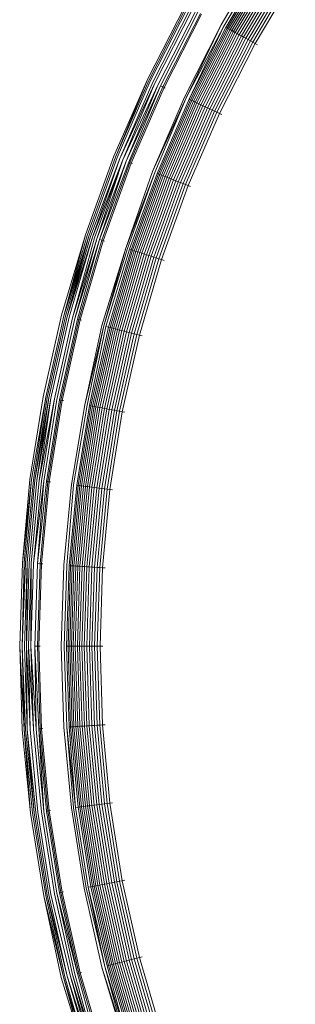
# Model space of a CAD drawing. Units: inches. Extents: x 64 to 1167, y 117 to 939.
# Tile 43 of 56: x 1129.1267 to 1129.3597, y 500.6393 to 501.4737. Entities that reach past the tile are written whole.
import ezdxf

# ---------------------------------------------------------------- set-up
doc = ezdxf.new("R2010")
doc.units = ezdxf.units.IN
doc.header["$MEASUREMENT"] = 0
doc.layers.add('A-FLOR-FIXT', color=8, linetype='Continuous', lineweight=18)

msp = doc.modelspace()

# ---------------------------------------------------------------- linework, layer by layer
at = {"layer": 'A-FLOR-FIXT'}
for p, q in [((1129.33193, 501.5286), (1129.29696, 501.46948)), ((1129.33413, 501.5272), (1129.29925, 501.46822)), ((1129.33586, 501.52611), (1129.30104, 501.46724)), ((1129.33689, 501.52546), (1129.30211, 501.46665)), ((1129.33802, 501.52474), (1129.30328, 501.466)), ((1129.33926, 501.52395), (1129.30457, 501.46529)), ((1129.34059, 501.52311), (1129.30595, 501.46453)), ((1129.34201, 501.5222), (1129.30743, 501.46372)), ((1129.34352, 501.52125), (1129.30899, 501.46286)), ((1129.34511, 501.52024), (1129.31064, 501.46196)), ((1129.34676, 501.51919), (1129.31236, 501.46101)), ((1129.34848, 501.5181), (1129.31414, 501.46003)), ((1129.35026, 501.51697), (1129.31599, 501.45902)), ((1129.35208, 501.51581), (1129.31788, 501.45798)), ((1129.35395, 501.51463), (1129.31982, 501.45691)), ((1129.35585, 501.51342), (1129.32179, 501.45583)), ((1129.35777, 501.5122), (1129.32378, 501.45473)), ((1129.35971, 501.51097), (1129.3258, 501.45362)), ((1129.2668, 501.48606), (1129.23464, 501.42293)), ((1129.26805, 501.48537), (1129.23593, 501.42232)), ((1129.26918, 501.48475), (1129.23709, 501.42177)), ((1129.27125, 501.48361), (1129.23923, 501.42076)), ((1129.27285, 501.48273), (1129.24089, 501.41999)), ((1129.27553, 501.48126), (1129.24365, 501.41869)), ((1129.27744, 501.48021), (1129.24562, 501.41776)), ((1129.27943, 501.47912), (1129.24767, 501.41679)), ((1129.28043, 501.47856), (1129.24871, 501.4163)), ((1129.29696, 501.46948), (1129.26598, 501.40818)), ((1129.29696, 501.46948), (1129.2674, 501.40751)), ((1129.29925, 501.46822), (1129.2674, 501.40751)), ((1129.29925, 501.46822), (1129.26998, 501.40629)), ((1129.30104, 501.46724), (1129.26998, 501.40629)), ((1129.30211, 501.46665), (1129.27109, 501.40577)), ((1129.30328, 501.466), (1129.27231, 501.4052)), ((1129.30457, 501.46529), (1129.27363, 501.40458)), ((1129.30595, 501.46453), (1129.27506, 501.4039)), ((1129.30211, 501.46665), (1129.30104, 501.46724)), ((1129.30328, 501.466), (1129.30211, 501.46665)), ((1129.30457, 501.46529), (1129.30328, 501.466)), ((1129.30595, 501.46453), (1129.30457, 501.46529)), ((1129.30743, 501.46372), (1129.30595, 501.46453)), ((1129.30743, 501.46372), (1129.27658, 501.40319)), ((1129.30899, 501.46286), (1129.2782, 501.40243)), ((1129.31064, 501.46196), (1129.2799, 501.40163)), ((1129.31236, 501.46101), (1129.28167, 501.40079)), ((1129.31414, 501.46003), (1129.28352, 501.39992)), ((1129.31599, 501.45902), (1129.28542, 501.39903)), ((1129.31788, 501.45798), (1129.28738, 501.39811)), ((1129.31982, 501.45691), (1129.28937, 501.39717)), ((1129.32179, 501.45583), (1129.29141, 501.39621)), ((1129.30899, 501.46286), (1129.30743, 501.46372)), ((1129.31064, 501.46196), (1129.30899, 501.46286)), ((1129.31236, 501.46101), (1129.31064, 501.46196)), ((1129.31414, 501.46003), (1129.31236, 501.46101)), ((1129.31599, 501.45902), (1129.31414, 501.46003)), ((1129.31788, 501.45798), (1129.31599, 501.45902)), ((1129.31982, 501.45691), (1129.31788, 501.45798)), ((1129.32179, 501.45583), (1129.31982, 501.45691)), ((1129.32378, 501.45473), (1129.32179, 501.45583)), ((1129.32378, 501.45473), (1129.29347, 501.39524)), ((1129.3258, 501.45362), (1129.29555, 501.39426)), ((1129.3258, 501.45362), (1129.32378, 501.45473)), ((1129.32782, 501.45251), (1129.3258, 501.45362)), ((1129.23464, 501.42293), (1129.20619, 501.35802)), ((1129.23464, 501.42293), (1129.20782, 501.35737)), ((1129.23593, 501.42232), (1129.20782, 501.35737)), ((1129.23709, 501.42177), (1129.20902, 501.3569)), ((1129.23923, 501.42076), (1129.21122, 501.35603)), ((1129.24089, 501.41999), (1129.21122, 501.35603)), ((1129.24089, 501.41999), (1129.21383, 501.355)), ((1129.24365, 501.41869), (1129.21383, 501.355)), ((1129.24365, 501.41869), (1129.21676, 501.35384)), ((1129.24562, 501.41776), (1129.21676, 501.35384)), ((1129.24562, 501.41776), (1129.21883, 501.35302)), ((1129.24767, 501.41679), (1129.21989, 501.3526)), ((1129.24871, 501.4163), (1129.22096, 501.35217)), ((1129.24767, 501.41679), (1129.24562, 501.41776)), ((1129.24767, 501.41679), (1129.24871, 501.4163)), ((1129.24871, 501.4163), (1129.24976, 501.41581)), ((1129.26598, 501.40818), (1129.23905, 501.34501)), ((1129.2674, 501.40751), (1129.23905, 501.34501)), ((1129.2674, 501.40751), (1129.24092, 501.34427)), ((1129.26998, 501.40629), (1129.24282, 501.34352)), ((1129.27109, 501.40577), (1129.24395, 501.34307)), ((1129.27109, 501.40577), (1129.26998, 501.40629)), ((1129.27231, 501.4052), (1129.27109, 501.40577)), ((1129.27231, 501.4052), (1129.2452, 501.34257)), ((1129.27363, 501.40458), (1129.24657, 501.34203)), ((1129.27506, 501.4039), (1129.24803, 501.34145)), ((1129.27658, 501.40319), (1129.2496, 501.34083)), ((1129.2782, 501.40243), (1129.25126, 501.34018)), ((1129.2799, 501.40163), (1129.25301, 501.33948)), ((1129.28167, 501.40079), (1129.25483, 501.33876)), ((1129.28352, 501.39992), (1129.25672, 501.33801)), ((1129.28542, 501.39903), (1129.25868, 501.33724)), ((1129.28738, 501.39811), (1129.26069, 501.33644)), ((1129.28937, 501.39717), (1129.26274, 501.33563)), ((1129.27363, 501.40458), (1129.27231, 501.4052)), ((1129.27506, 501.4039), (1129.27363, 501.40458)), ((1129.27658, 501.40319), (1129.27506, 501.4039)), ((1129.2782, 501.40243), (1129.27658, 501.40319)), ((1129.2799, 501.40163), (1129.2782, 501.40243)), ((1129.28167, 501.40079), (1129.2799, 501.40163)), ((1129.28352, 501.39992), (1129.28167, 501.40079)), ((1129.28542, 501.39903), (1129.28352, 501.39992)), ((1129.28738, 501.39811), (1129.28542, 501.39903)), ((1129.28937, 501.39717), (1129.28738, 501.39811)), ((1129.29141, 501.39621), (1129.28937, 501.39717)), ((1129.29141, 501.39621), (1129.26484, 501.3348)), ((1129.29347, 501.39524), (1129.26695, 501.33396)), ((1129.29555, 501.39426), (1129.26909, 501.33312)), ((1129.29347, 501.39524), (1129.29141, 501.39621)), ((1129.29555, 501.39426), (1129.29347, 501.39524)), ((1129.29764, 501.39328), (1129.29555, 501.39426)), ((1129.20619, 501.35802), (1129.18218, 501.29134)), ((1129.20782, 501.35737), (1129.18385, 501.29079)), ((1129.20902, 501.3569), (1129.18507, 501.2904)), ((1129.21122, 501.35603), (1129.18652, 501.28993)), ((1129.21122, 501.35603), (1129.18817, 501.28939)), ((1129.21383, 501.355), (1129.18817, 501.28939)), ((1129.21383, 501.355), (1129.19, 501.2888)), ((1129.21383, 501.355), (1129.19197, 501.28816)), ((1129.21676, 501.35384), (1129.19197, 501.28816)), ((1129.21676, 501.35384), (1129.19404, 501.28748)), ((1129.21883, 501.35302), (1129.19404, 501.28748)), ((1129.21989, 501.3526), (1129.1962, 501.28678)), ((1129.22096, 501.35217), (1129.19729, 501.28643)), ((1129.21883, 501.35302), (1129.21989, 501.3526)), ((1129.21989, 501.3526), (1129.22096, 501.35217)), ((1129.22096, 501.35217), (1129.22203, 501.35175)), ((1129.23905, 501.34501), (1129.2163, 501.28025)), ((1129.24092, 501.34427), (1129.2163, 501.28025)), ((1129.24092, 501.34427), (1129.21771, 501.27979)), ((1129.24282, 501.34352), (1129.21965, 501.27916)), ((1129.24395, 501.34307), (1129.22081, 501.27879)), ((1129.2452, 501.34257), (1129.22209, 501.27837)), ((1129.24657, 501.34203), (1129.22348, 501.27792)), ((1129.24803, 501.34145), (1129.22498, 501.27743)), ((1129.2496, 501.34083), (1129.22659, 501.27691)), ((1129.25126, 501.34018), (1129.22829, 501.27636)), ((1129.25301, 501.33948), (1129.23007, 501.27578)), ((1129.25483, 501.33876), (1129.23194, 501.27517)), ((1129.24282, 501.34352), (1129.24395, 501.34307)), ((1129.24395, 501.34307), (1129.2452, 501.34257)), ((1129.2452, 501.34257), (1129.24657, 501.34203)), ((1129.24657, 501.34203), (1129.24803, 501.34145)), ((1129.24803, 501.34145), (1129.2496, 501.34083)), ((1129.2496, 501.34083), (1129.25126, 501.34018)), ((1129.25126, 501.34018), (1129.25301, 501.33948)), ((1129.25301, 501.33948), (1129.25483, 501.33876)), ((1129.25483, 501.33876), (1129.25672, 501.33801)), ((1129.25672, 501.33801), (1129.23387, 501.27454)), ((1129.25868, 501.33724), (1129.23587, 501.27389)), ((1129.26069, 501.33644), (1129.23793, 501.27322)), ((1129.26274, 501.33563), (1129.24003, 501.27254)), ((1129.26484, 501.3348), (1129.24217, 501.27185)), ((1129.26695, 501.33396), (1129.24434, 501.27114)), ((1129.26909, 501.33312), (1129.24652, 501.27043)), ((1129.25672, 501.33801), (1129.25868, 501.33724)), ((1129.25868, 501.33724), (1129.26069, 501.33644)), ((1129.26069, 501.33644), (1129.26274, 501.33563)), ((1129.26274, 501.33563), (1129.26484, 501.3348)), ((1129.26484, 501.3348), (1129.26695, 501.33396)), ((1129.26695, 501.33396), (1129.26909, 501.33312)), ((1129.26909, 501.33312), (1129.27124, 501.33227)), ((1129.18218, 501.29134), (1129.16197, 501.22339)), ((1129.18218, 501.29134), (1129.16411, 501.22284)), ((1129.18385, 501.29079), (1129.16411, 501.22284)), ((1129.18507, 501.2904), (1129.16411, 501.22284)), ((1129.18507, 501.2904), (1129.16535, 501.22252)), ((1129.18507, 501.2904), (1129.16683, 501.22214)), ((1129.18652, 501.28993), (1129.16683, 501.22214)), ((1129.18817, 501.28939), (1129.16683, 501.22214)), ((1129.18817, 501.28939), (1129.16851, 501.22171)), ((1129.19, 501.2888), (1129.17135, 501.22098)), ((1129.19197, 501.28816), (1129.17135, 501.22098)), ((1129.19197, 501.28816), (1129.17342, 501.22045)), ((1129.19404, 501.28748), (1129.17342, 501.22045)), ((1129.19404, 501.28748), (1129.17558, 501.21989)), ((1129.1962, 501.28678), (1129.17668, 501.21961)), ((1129.19729, 501.28643), (1129.1778, 501.21933)), ((1129.1962, 501.28678), (1129.19404, 501.28748)), ((1129.19729, 501.28643), (1129.1962, 501.28678)), ((1129.19839, 501.28607), (1129.19729, 501.28643)), ((1129.2163, 501.28025), (1129.19606, 501.21464)), ((1129.2163, 501.28025), (1129.1978, 501.21419)), ((1129.21771, 501.27979), (1129.1978, 501.21419)), ((1129.21965, 501.27916), (1129.19951, 501.21375)), ((1129.22081, 501.27879), (1129.20175, 501.21318)), ((1129.22209, 501.27837), (1129.20305, 501.21284)), ((1129.22348, 501.27792), (1129.20447, 501.21248)), ((1129.22498, 501.27743), (1129.206, 501.21208)), ((1129.22659, 501.27691), (1129.20763, 501.21166)), ((1129.22829, 501.27636), (1129.20936, 501.21122)), ((1129.23007, 501.27578), (1129.21118, 501.21075)), ((1129.23194, 501.27517), (1129.21308, 501.21027)), ((1129.23387, 501.27454), (1129.21505, 501.20976)), ((1129.23587, 501.27389), (1129.21709, 501.20924)), ((1129.23793, 501.27322), (1129.21918, 501.2087)), ((1129.22081, 501.27879), (1129.21965, 501.27916)), ((1129.22209, 501.27837), (1129.22081, 501.27879)), ((1129.24003, 501.27254), (1129.22132, 501.20815)), ((1129.22348, 501.27792), (1129.22209, 501.27837)), ((1129.22498, 501.27743), (1129.22348, 501.27792)), ((1129.22659, 501.27691), (1129.22498, 501.27743)), ((1129.22829, 501.27636), (1129.22659, 501.27691)), ((1129.23007, 501.27578), (1129.22829, 501.27636)), ((1129.23194, 501.27517), (1129.23007, 501.27578)), ((1129.23387, 501.27454), (1129.23194, 501.27517)), ((1129.23587, 501.27389), (1129.23387, 501.27454)), ((1129.23793, 501.27322), (1129.23587, 501.27389)), ((1129.24003, 501.27254), (1129.23793, 501.27322)), ((1129.24217, 501.27185), (1129.24003, 501.27254)), ((1129.24217, 501.27185), (1129.2235, 501.20759)), ((1129.24434, 501.27114), (1129.22571, 501.20702)), ((1129.24652, 501.27043), (1129.22794, 501.20645)), ((1129.24434, 501.27114), (1129.24217, 501.27185)), ((1129.24652, 501.27043), (1129.24434, 501.27114)), ((1129.24872, 501.26972), (1129.24652, 501.27043)), ((1129.16197, 501.22339), (1129.1465, 501.15419)), ((1129.16411, 501.22284), (1129.14867, 501.15378)), ((1129.16535, 501.22252), (1129.14993, 501.15354)), ((1129.16683, 501.22214), (1129.15143, 501.15325)), ((1129.16851, 501.22171), (1129.15313, 501.15293)), ((1129.17135, 501.22098), (1129.15602, 501.15238)), ((1129.17342, 501.22045), (1129.15811, 501.15198)), ((1129.17558, 501.21989), (1129.1603, 501.15156)), ((1129.17668, 501.21961), (1129.16142, 501.15135)), ((1129.1778, 501.21933), (1129.16255, 501.15113)), ((1129.17668, 501.21961), (1129.17558, 501.21989)), ((1129.1778, 501.21933), (1129.17668, 501.21961)), ((1129.17891, 501.21904), (1129.1778, 501.21933)), ((1129.19606, 501.21464), (1129.18167, 501.14749)), ((1129.1978, 501.21419), (1129.18167, 501.14749)), ((1129.1978, 501.21419), (1129.18364, 501.14711)), ((1129.19951, 501.21375), (1129.18565, 501.14673)), ((1129.20175, 501.21318), (1129.19951, 501.21375)), ((1129.20175, 501.21318), (1129.18684, 501.1465)), ((1129.20305, 501.21284), (1129.18817, 501.14625)), ((1129.20447, 501.21248), (1129.18961, 501.14597)), ((1129.206, 501.21208), (1129.19116, 501.14568)), ((1129.20763, 501.21166), (1129.19281, 501.14536)), ((1129.20936, 501.21122), (1129.19457, 501.14503)), ((1129.21118, 501.21075), (1129.19641, 501.14467)), ((1129.21308, 501.21027), (1129.19834, 501.14431)), ((1129.21505, 501.20976), (1129.20034, 501.14392)), ((1129.20305, 501.21284), (1129.20175, 501.21318)), ((1129.21709, 501.20924), (1129.2024, 501.14353)), ((1129.20447, 501.21248), (1129.20305, 501.21284)), ((1129.206, 501.21208), (1129.20447, 501.21248)), ((1129.21918, 501.2087), (1129.20453, 501.14313)), ((1129.20763, 501.21166), (1129.206, 501.21208)), ((1129.22132, 501.20815), (1129.2067, 501.14271)), ((1129.20936, 501.21122), (1129.20763, 501.21166)), ((1129.2235, 501.20759), (1129.20891, 501.14229)), ((1129.21118, 501.21075), (1129.20936, 501.21122)), ((1129.22571, 501.20702), (1129.21114, 501.14186)), ((1129.21308, 501.21027), (1129.21118, 501.21075)), ((1129.21505, 501.20976), (1129.21308, 501.21027)), ((1129.22794, 501.20645), (1129.2134, 501.14143)), ((1129.21709, 501.20924), (1129.21505, 501.20976)), ((1129.21918, 501.2087), (1129.21709, 501.20924)), ((1129.22132, 501.20815), (1129.21918, 501.2087)), ((1129.2235, 501.20759), (1129.22132, 501.20815)), ((1129.22571, 501.20702), (1129.2235, 501.20759)), ((1129.22794, 501.20645), (1129.22571, 501.20702)), ((1129.23017, 501.20588), (1129.22794, 501.20645)), ((1129.1465, 501.15419), (1129.1353, 501.08418)), ((1129.14867, 501.15378), (1129.13659, 501.08401)), ((1129.14867, 501.15378), (1129.13821, 501.08381)), ((1129.14993, 501.15354), (1129.1396, 501.08363)), ((1129.15143, 501.15325), (1129.1396, 501.08363)), ((1129.15143, 501.15325), (1129.14122, 501.08343)), ((1129.15313, 501.15293), (1129.14122, 501.08343)), ((1129.15313, 501.15293), (1129.14304, 501.0832)), ((1129.15602, 501.15238), (1129.14304, 501.0832)), ((1129.15602, 501.15238), (1129.14502, 501.08295)), ((1129.15811, 501.15198), (1129.14714, 501.08268)), ((1129.1603, 501.15156), (1129.14935, 501.0824)), ((1129.16142, 501.15135), (1129.15048, 501.08226)), ((1129.16255, 501.15113), (1129.15162, 501.08212)), ((1129.1603, 501.15156), (1129.16142, 501.15135)), ((1129.16142, 501.15135), (1129.16255, 501.15113)), ((1129.16255, 501.15113), (1129.16369, 501.15092)), ((1129.18167, 501.14749), (1129.17056, 501.07972)), ((1129.18364, 501.14711), (1129.17211, 501.07953)), ((1129.18565, 501.14673), (1129.17495, 501.07917)), ((1129.18684, 501.1465), (1129.17616, 501.07902)), ((1129.18817, 501.14625), (1129.17749, 501.07885)), ((1129.18961, 501.14597), (1129.17894, 501.07866)), ((1129.19116, 501.14568), (1129.18051, 501.07847)), ((1129.19281, 501.14536), (1129.18218, 501.07825)), ((1129.19457, 501.14503), (1129.18395, 501.07803)), ((1129.18684, 501.1465), (1129.18565, 501.14673)), ((1129.19641, 501.14467), (1129.18582, 501.0778)), ((1129.18817, 501.14625), (1129.18684, 501.1465)), ((1129.19834, 501.14431), (1129.18776, 501.07755)), ((1129.18961, 501.14597), (1129.18817, 501.14625)), ((1129.19116, 501.14568), (1129.18961, 501.14597)), ((1129.20034, 501.14392), (1129.18978, 501.07729)), ((1129.19281, 501.14536), (1129.19116, 501.14568)), ((1129.2024, 501.14353), (1129.19187, 501.07703)), ((1129.19457, 501.14503), (1129.19281, 501.14536)), ((1129.20453, 501.14313), (1129.19401, 501.07676)), ((1129.19641, 501.14467), (1129.19457, 501.14503)), ((1129.2067, 501.14271), (1129.19621, 501.07648)), ((1129.19834, 501.14431), (1129.19641, 501.14467)), ((1129.20034, 501.14392), (1129.19834, 501.14431)), ((1129.20891, 501.14229), (1129.19844, 501.0762)), ((1129.2024, 501.14353), (1129.20034, 501.14392)), ((1129.21114, 501.14186), (1129.2007, 501.07592)), ((1129.20453, 501.14313), (1129.2024, 501.14353)), ((1129.2134, 501.14143), (1129.20298, 501.07563)), ((1129.2067, 501.14271), (1129.20453, 501.14313)), ((1129.20891, 501.14229), (1129.2067, 501.14271)), ((1129.21114, 501.14186), (1129.20891, 501.14229)), ((1129.2134, 501.14143), (1129.21114, 501.14186)), ((1129.21567, 501.141), (1129.2134, 501.14143)), ((1129.1353, 501.08418), (1129.12892, 501.01356)), ((1129.13659, 501.08401), (1129.12892, 501.01356)), ((1129.13659, 501.08401), (1129.1304, 501.01347)), ((1129.13821, 501.08381), (1129.13155, 501.0134)), ((1129.1396, 501.08363), (1129.13296, 501.01331)), ((1129.14122, 501.08343), (1129.13459, 501.01321)), ((1129.14304, 501.0832), (1129.13641, 501.01309)), ((1129.14502, 501.08295), (1129.13841, 501.01297)), ((1129.14714, 501.08268), (1129.13841, 501.01297)), ((1129.14714, 501.08268), (1129.14164, 501.01276)), ((1129.14935, 501.0824), (1129.14164, 501.01276)), ((1129.15048, 501.08226), (1129.1439, 501.01262)), ((1129.15162, 501.08212), (1129.14505, 501.01255)), ((1129.15048, 501.08226), (1129.14935, 501.0824)), ((1129.15162, 501.08212), (1129.15048, 501.08226)), ((1129.15277, 501.08197), (1129.15162, 501.08212)), ((1129.17056, 501.07972), (1129.16409, 501.01135)), ((1129.17211, 501.07953), (1129.16647, 501.0112)), ((1129.17495, 501.07917), (1129.16851, 501.01107)), ((1129.17616, 501.07902), (1129.16973, 501.011)), ((1129.17749, 501.07885), (1129.17107, 501.01091)), ((1129.17894, 501.07866), (1129.17253, 501.01082)), ((1129.18051, 501.07847), (1129.17411, 501.01072)), ((1129.17616, 501.07902), (1129.17495, 501.07917)), ((1129.18218, 501.07825), (1129.17579, 501.01062)), ((1129.17749, 501.07885), (1129.17616, 501.07902)), ((1129.17894, 501.07866), (1129.17749, 501.07885)), ((1129.18395, 501.07803), (1129.17757, 501.0105)), ((1129.18051, 501.07847), (1129.17894, 501.07866)), ((1129.18582, 501.0778), (1129.17944, 501.01039)), ((1129.18218, 501.07825), (1129.18051, 501.07847)), ((1129.18776, 501.07755), (1129.1814, 501.01026)), ((1129.18395, 501.07803), (1129.18218, 501.07825)), ((1129.18978, 501.07729), (1129.18344, 501.01013)), ((1129.18582, 501.0778), (1129.18395, 501.07803)), ((1129.19187, 501.07703), (1129.18553, 501.01)), ((1129.18776, 501.07755), (1129.18582, 501.0778)), ((1129.19401, 501.07676), (1129.18769, 501.00987)), ((1129.18978, 501.07729), (1129.18776, 501.07755)), ((1129.19187, 501.07703), (1129.18978, 501.07729)), ((1129.19621, 501.07648), (1129.1899, 501.00973)), ((1129.19187, 501.07703), (1129.19401, 501.07676)), ((1129.19844, 501.0762), (1129.19214, 501.00959)), ((1129.19401, 501.07676), (1129.19621, 501.07648)), ((1129.2007, 501.07592), (1129.19442, 501.00944)), ((1129.19621, 501.07648), (1129.19844, 501.0762)), ((1129.20298, 501.07563), (1129.19671, 501.0093)), ((1129.19844, 501.0762), (1129.2007, 501.07592)), ((1129.2007, 501.07592), (1129.20298, 501.07563)), ((1129.20298, 501.07563), (1129.20527, 501.07534)), ((1129.12892, 501.01356), (1129.1267, 500.94271)), ((1129.1304, 501.01347), (1129.12872, 500.94271)), ((1129.13155, 501.0134), (1129.12872, 500.94271)), ((1129.13296, 501.01331), (1129.13074, 500.94271)), ((1129.13296, 501.01331), (1129.13237, 500.94271)), ((1129.13459, 501.01321), (1129.13237, 500.94271)), ((1129.13641, 501.01309), (1129.1342, 500.94271)), ((1129.13641, 501.01309), (1129.1362, 500.94271)), ((1129.13841, 501.01297), (1129.1362, 500.94271)), ((1129.14164, 501.01276), (1129.13944, 500.94271)), ((1129.14164, 501.01276), (1129.1439, 501.01262)), ((1129.1439, 501.01262), (1129.1417, 500.94271)), ((1129.14505, 501.01255), (1129.14285, 500.94271)), ((1129.1439, 501.01262), (1129.14505, 501.01255)), ((1129.14505, 501.01255), (1129.1462, 501.01248)), ((1129.16409, 501.01135), (1129.16171, 500.94271)), ((1129.16647, 501.0112), (1129.16432, 500.94271)), ((1129.16851, 501.01107), (1129.16636, 500.94271)), ((1129.16973, 501.011), (1129.16758, 500.94271)), ((1129.16973, 501.011), (1129.16851, 501.01107)), ((1129.17107, 501.01091), (1129.16893, 500.94271)), ((1129.17107, 501.01091), (1129.16973, 501.011)), ((1129.17253, 501.01082), (1129.17039, 500.94271)), ((1129.17253, 501.01082), (1129.17107, 501.01091)), ((1129.17411, 501.01072), (1129.17197, 500.94271)), ((1129.17411, 501.01072), (1129.17253, 501.01082)), ((1129.17579, 501.01062), (1129.17366, 500.94271)), ((1129.17579, 501.01062), (1129.17411, 501.01072)), ((1129.17757, 501.0105), (1129.17544, 500.94271)), ((1129.17757, 501.0105), (1129.17579, 501.01062)), ((1129.17944, 501.01039), (1129.17732, 500.94271)), ((1129.17944, 501.01039), (1129.17757, 501.0105)), ((1129.1814, 501.01026), (1129.17928, 500.94271)), ((1129.1814, 501.01026), (1129.17944, 501.01039)), ((1129.18344, 501.01013), (1129.18132, 500.94271)), ((1129.18344, 501.01013), (1129.1814, 501.01026)), ((1129.18553, 501.01), (1129.18342, 500.94271)), ((1129.18553, 501.01), (1129.18344, 501.01013)), ((1129.18769, 501.00987), (1129.18553, 501.01)), ((1129.18769, 501.00987), (1129.18558, 500.94271)), ((1129.1899, 501.00973), (1129.18769, 501.00987)), ((1129.1899, 501.00973), (1129.18779, 500.94271)), ((1129.19214, 501.00959), (1129.1899, 501.00973)), ((1129.19214, 501.00959), (1129.19004, 500.94271)), ((1129.19442, 501.00944), (1129.19214, 501.00959)), ((1129.19442, 501.00944), (1129.19232, 500.94271)), ((1129.19671, 501.0093), (1129.19442, 501.00944)), ((1129.19671, 501.0093), (1129.19462, 500.94271)), ((1129.19901, 501.00915), (1129.19671, 501.0093)), ((1129.1267, 500.94271), (1129.1304, 500.87194)), ((1129.1267, 500.94271), (1129.12874, 500.87184)), ((1129.12872, 500.94271), (1129.1304, 500.87194)), ((1129.12872, 500.94271), (1129.13155, 500.87202)), ((1129.13074, 500.94271), (1129.13296, 500.87211)), ((1129.13237, 500.94271), (1129.13548, 500.87226)), ((1129.13237, 500.94271), (1129.13296, 500.87211)), ((1129.1342, 500.94271), (1129.13841, 500.87245)), ((1129.1342, 500.94271), (1129.13548, 500.87226)), ((1129.1362, 500.94271), (1129.14054, 500.87258)), ((1129.1362, 500.94271), (1129.13841, 500.87245)), ((1129.1417, 500.94271), (1129.13944, 500.94271)), ((1129.13944, 500.94271), (1129.14276, 500.87272)), ((1129.13944, 500.94271), (1129.14054, 500.87258)), ((1129.14285, 500.94271), (1129.1417, 500.94271)), ((1129.1417, 500.94271), (1129.1439, 500.87279)), ((1129.144, 500.94271), (1129.14285, 500.94271)), ((1129.14285, 500.94271), (1129.14505, 500.87287)), ((1129.16171, 500.94271), (1129.16387, 500.87405)), ((1129.16432, 500.94271), (1129.16647, 500.87421)), ((1129.16636, 500.94271), (1129.16758, 500.94271)), ((1129.16636, 500.94271), (1129.16851, 500.87434)), ((1129.16758, 500.94271), (1129.16893, 500.94271)), ((1129.16758, 500.94271), (1129.16973, 500.87442)), ((1129.16893, 500.94271), (1129.17039, 500.94271)), ((1129.16893, 500.94271), (1129.17107, 500.8745)), ((1129.17039, 500.94271), (1129.17197, 500.94271)), ((1129.17039, 500.94271), (1129.17253, 500.8746)), ((1129.17197, 500.94271), (1129.17366, 500.94271)), ((1129.17197, 500.94271), (1129.17411, 500.87469)), ((1129.17366, 500.94271), (1129.17544, 500.94271)), ((1129.17366, 500.94271), (1129.17579, 500.8748)), ((1129.17544, 500.94271), (1129.17732, 500.94271)), ((1129.17544, 500.94271), (1129.17757, 500.87491)), ((1129.17732, 500.94271), (1129.17928, 500.94271)), ((1129.17732, 500.94271), (1129.17944, 500.87503)), ((1129.17928, 500.94271), (1129.18132, 500.94271)), ((1129.17928, 500.94271), (1129.1814, 500.87515)), ((1129.18132, 500.94271), (1129.18342, 500.94271)), ((1129.18132, 500.94271), (1129.18344, 500.87528)), ((1129.18342, 500.94271), (1129.18558, 500.94271)), ((1129.18342, 500.94271), (1129.18553, 500.87541)), ((1129.18558, 500.94271), (1129.18769, 500.87555)), ((1129.18558, 500.94271), (1129.18779, 500.94271)), ((1129.18779, 500.94271), (1129.19004, 500.94271)), ((1129.18779, 500.94271), (1129.1899, 500.87569)), ((1129.19004, 500.94271), (1129.19232, 500.94271)), ((1129.19004, 500.94271), (1129.19214, 500.87583)), ((1129.19232, 500.94271), (1129.19462, 500.94271)), ((1129.19232, 500.94271), (1129.19442, 500.87597)), ((1129.19462, 500.94271), (1129.19693, 500.94271)), ((1129.19462, 500.94271), (1129.19671, 500.87612)), ((1129.12874, 500.87184), (1129.13586, 500.80131)), ((1129.1304, 500.87194), (1129.1376, 500.80153)), ((1129.1304, 500.87194), (1129.13586, 500.80131)), ((1129.13155, 500.87202), (1129.13888, 500.80169)), ((1129.13296, 500.87211), (1129.13888, 500.80169)), ((1129.13296, 500.87211), (1129.14039, 500.80188)), ((1129.13548, 500.87226), (1129.14211, 500.8021)), ((1129.13841, 500.87245), (1129.14502, 500.80247)), ((1129.14054, 500.87258), (1129.14714, 500.80273)), ((1129.14276, 500.87272), (1129.1439, 500.87279)), ((1129.14276, 500.87272), (1129.14935, 500.80301)), ((1129.14276, 500.87272), (1129.14714, 500.80273)), ((1129.1439, 500.87279), (1129.14505, 500.87287)), ((1129.1439, 500.87279), (1129.15048, 500.80316)), ((1129.14505, 500.87287), (1129.1462, 500.87294)), ((1129.14505, 500.87287), (1129.15162, 500.8033)), ((1129.16387, 500.87405), (1129.17056, 500.80569)), ((1129.16647, 500.87421), (1129.17387, 500.80611)), ((1129.16647, 500.87421), (1129.17211, 500.80589)), ((1129.16973, 500.87442), (1129.16851, 500.87434)), ((1129.16851, 500.87434), (1129.17387, 500.80611)), ((1129.17107, 500.8745), (1129.16973, 500.87442)), ((1129.16973, 500.87442), (1129.17616, 500.8064)), ((1129.17253, 500.8746), (1129.17107, 500.8745)), ((1129.17107, 500.8745), (1129.17749, 500.80657)), ((1129.17411, 500.87469), (1129.17253, 500.8746)), ((1129.17253, 500.8746), (1129.17894, 500.80675)), ((1129.17579, 500.8748), (1129.17411, 500.87469)), ((1129.17411, 500.87469), (1129.18051, 500.80695)), ((1129.17757, 500.87491), (1129.17579, 500.8748)), ((1129.17579, 500.8748), (1129.18218, 500.80716)), ((1129.17944, 500.87503), (1129.17757, 500.87491)), ((1129.17757, 500.87491), (1129.18395, 500.80738)), ((1129.1814, 500.87515), (1129.17944, 500.87503)), ((1129.17944, 500.87503), (1129.18582, 500.80762)), ((1129.18344, 500.87528), (1129.1814, 500.87515)), ((1129.1814, 500.87515), (1129.18776, 500.80787)), ((1129.18553, 500.87541), (1129.18344, 500.87528)), ((1129.18344, 500.87528), (1129.18978, 500.80812)), ((1129.18769, 500.87555), (1129.18553, 500.87541)), ((1129.18553, 500.87541), (1129.19187, 500.80838)), ((1129.1899, 500.87569), (1129.18769, 500.87555)), ((1129.18769, 500.87555), (1129.19401, 500.80865)), ((1129.19214, 500.87583), (1129.1899, 500.87569)), ((1129.1899, 500.87569), (1129.19621, 500.80893)), ((1129.19442, 500.87597), (1129.19214, 500.87583)), ((1129.19214, 500.87583), (1129.19844, 500.80921)), ((1129.19671, 500.87612), (1129.19442, 500.87597)), ((1129.19442, 500.87597), (1129.2007, 500.8095)), ((1129.19901, 500.87626), (1129.19671, 500.87612)), ((1129.19671, 500.87612), (1129.20298, 500.80979)), ((1129.17056, 500.80569), (1129.18108, 500.73782)), ((1129.17211, 500.80589), (1129.18284, 500.73815)), ((1129.17616, 500.8064), (1129.17387, 500.80611)), ((1129.17387, 500.80611), (1129.18458, 500.73848)), ((1129.17749, 500.80657), (1129.17616, 500.8064)), ((1129.17616, 500.8064), (1129.18684, 500.73892)), ((1129.17894, 500.80675), (1129.17749, 500.80657)), ((1129.17749, 500.80657), (1129.18817, 500.73917)), ((1129.18051, 500.80695), (1129.17894, 500.80675)), ((1129.17894, 500.80675), (1129.18961, 500.73944)), ((1129.18218, 500.80716), (1129.18051, 500.80695)), ((1129.18051, 500.80695), (1129.19116, 500.73974)), ((1129.18395, 500.80738), (1129.18218, 500.80716)), ((1129.18218, 500.80716), (1129.19281, 500.74006)), ((1129.18582, 500.80762), (1129.18395, 500.80738)), ((1129.18395, 500.80738), (1129.19457, 500.74039)), ((1129.18776, 500.80787), (1129.18582, 500.80762)), ((1129.18582, 500.80762), (1129.19641, 500.74074)), ((1129.18978, 500.80812), (1129.18776, 500.80787)), ((1129.18776, 500.80787), (1129.19834, 500.74111)), ((1129.19187, 500.80838), (1129.18978, 500.80812)), ((1129.18978, 500.80812), (1129.20034, 500.74149)), ((1129.19401, 500.80865), (1129.19187, 500.80838)), ((1129.19187, 500.80838), (1129.2024, 500.74189)), ((1129.19621, 500.80893), (1129.19401, 500.80865)), ((1129.19401, 500.80865), (1129.20453, 500.74229)), ((1129.19844, 500.80921), (1129.19621, 500.80893)), ((1129.19621, 500.80893), (1129.2067, 500.7427)), ((1129.2007, 500.8095), (1129.19844, 500.80921)), ((1129.19844, 500.80921), (1129.20891, 500.74313)), ((1129.20298, 500.80979), (1129.2007, 500.8095)), ((1129.2007, 500.8095), (1129.21114, 500.74355)), ((1129.20527, 500.81008), (1129.20298, 500.80979)), ((1129.20298, 500.80979), (1129.2134, 500.74398)), ((1129.13586, 500.80131), (1129.14694, 500.73131)), ((1129.1376, 500.80153), (1129.14867, 500.73164)), ((1129.13888, 500.80169), (1129.14993, 500.73188)), ((1129.14039, 500.80188), (1129.15143, 500.73216)), ((1129.14211, 500.8021), (1129.15313, 500.73249)), ((1129.14502, 500.80247), (1129.15602, 500.73304)), ((1129.14714, 500.80273), (1129.15811, 500.73344)), ((1129.15048, 500.80316), (1129.14935, 500.80301)), ((1129.14935, 500.80301), (1129.1603, 500.73385)), ((1129.15162, 500.8033), (1129.15048, 500.80316)), ((1129.15048, 500.80316), (1129.16142, 500.73407)), ((1129.15277, 500.80344), (1129.15162, 500.8033)), ((1129.15162, 500.8033), (1129.16255, 500.73428)), ((1129.18284, 500.73815), (1129.19859, 500.67143)), ((1129.18684, 500.73892), (1129.18458, 500.73848)), ((1129.18458, 500.73848), (1129.20057, 500.67194)), ((1129.18458, 500.73848), (1129.19859, 500.67143)), ((1129.18817, 500.73917), (1129.18684, 500.73892)), ((1129.18684, 500.73892), (1129.20175, 500.67224)), ((1129.18961, 500.73944), (1129.18817, 500.73917)), ((1129.18817, 500.73917), (1129.20305, 500.67257)), ((1129.19116, 500.73974), (1129.18961, 500.73944)), ((1129.18961, 500.73944), (1129.20447, 500.67294)), ((1129.19281, 500.74006), (1129.19116, 500.73974)), ((1129.19116, 500.73974), (1129.206, 500.67333)), ((1129.19457, 500.74039), (1129.19281, 500.74006)), ((1129.19281, 500.74006), (1129.20763, 500.67375)), ((1129.19641, 500.74074), (1129.19457, 500.74039)), ((1129.19457, 500.74039), (1129.20936, 500.67419)), ((1129.19834, 500.74111), (1129.19641, 500.74074)), ((1129.19641, 500.74074), (1129.21118, 500.67466)), ((1129.20034, 500.74149), (1129.19834, 500.74111)), ((1129.19834, 500.74111), (1129.21308, 500.67515)), ((1129.2024, 500.74189), (1129.20034, 500.74149)), ((1129.20034, 500.74149), (1129.21505, 500.67566)), ((1129.20453, 500.74229), (1129.2024, 500.74189)), ((1129.2024, 500.74189), (1129.21709, 500.67618)), ((1129.2067, 500.7427), (1129.20453, 500.74229)), ((1129.20453, 500.74229), (1129.21918, 500.67672)), ((1129.20891, 500.74313), (1129.2067, 500.7427)), ((1129.2067, 500.7427), (1129.22132, 500.67727)), ((1129.21114, 500.74355), (1129.20891, 500.74313)), ((1129.20891, 500.74313), (1129.2235, 500.67783)), ((1129.2134, 500.74398), (1129.21114, 500.74355)), ((1129.21114, 500.74355), (1129.22571, 500.67839)), ((1129.21567, 500.74442), (1129.2134, 500.74398)), ((1129.2134, 500.74398), (1129.22794, 500.67896)), ((1129.14694, 500.73131), (1129.16358, 500.66244)), ((1129.14694, 500.73131), (1129.16182, 500.66199)), ((1129.14867, 500.73164), (1129.16358, 500.66244)), ((1129.14993, 500.73188), (1129.16683, 500.66327)), ((1129.14993, 500.73188), (1129.1647, 500.66273)), ((1129.15143, 500.73216), (1129.16683, 500.66327)), ((1129.15313, 500.73249), (1129.16942, 500.66394)), ((1129.15602, 500.73304), (1129.17135, 500.66444)), ((1129.15811, 500.73344), (1129.17558, 500.66552)), ((1129.15811, 500.73344), (1129.17342, 500.66497)), ((1129.1603, 500.73385), (1129.16142, 500.73407)), ((1129.1603, 500.73385), (1129.17558, 500.66552)), ((1129.16142, 500.73407), (1129.16255, 500.73428)), ((1129.16142, 500.73407), (1129.17668, 500.6658)), ((1129.16255, 500.73428), (1129.16369, 500.7345)), ((1129.16255, 500.73428), (1129.1778, 500.66609)), ((1129.18108, 500.73782), (1129.19606, 500.67078)), ((1129.19859, 500.67143), (1129.21862, 500.60592)), ((1129.19859, 500.67143), (1129.21694, 500.60537)), ((1129.20175, 500.67224), (1129.20057, 500.67194)), ((1129.20057, 500.67194), (1129.21862, 500.60592)), ((1129.20305, 500.67257), (1129.20175, 500.67224)), ((1129.20175, 500.67224), (1129.22081, 500.60663)), ((1129.20447, 500.67294), (1129.20305, 500.67257)), ((1129.20305, 500.67257), (1129.22209, 500.60705)), ((1129.206, 500.67333), (1129.20447, 500.67294)), ((1129.20447, 500.67294), (1129.22348, 500.6075)), ((1129.20763, 500.67375), (1129.206, 500.67333)), ((1129.206, 500.67333), (1129.22498, 500.60799)), ((1129.20936, 500.67419), (1129.20763, 500.67375)), ((1129.20763, 500.67375), (1129.22659, 500.60851)), ((1129.21118, 500.67466), (1129.20936, 500.67419)), ((1129.20936, 500.67419), (1129.22829, 500.60906)), ((1129.21308, 500.67515), (1129.21118, 500.67466)), ((1129.21118, 500.67466), (1129.23007, 500.60964)), ((1129.21505, 500.67566), (1129.21308, 500.67515)), ((1129.21308, 500.67515), (1129.23194, 500.61024)), ((1129.21709, 500.67618), (1129.21505, 500.67566)), ((1129.21505, 500.67566), (1129.23387, 500.61087)), ((1129.21918, 500.67672), (1129.21709, 500.67618)), ((1129.21709, 500.67618), (1129.23587, 500.61152)), ((1129.22132, 500.67727), (1129.21918, 500.67672)), ((1129.21918, 500.67672), (1129.23793, 500.61219)), ((1129.2235, 500.67783), (1129.22132, 500.67727)), ((1129.22132, 500.67727), (1129.24003, 500.61288)), ((1129.22571, 500.67839), (1129.2235, 500.67783)), ((1129.2235, 500.67783), (1129.24217, 500.61357)), ((1129.22794, 500.67896), (1129.22571, 500.67839)), ((1129.22571, 500.67839), (1129.24434, 500.61427)), ((1129.23017, 500.67954), (1129.22794, 500.67896)), ((1129.22794, 500.67896), (1129.24652, 500.61498)), ((1129.16683, 500.66327), (1129.18817, 500.59602)), ((1129.16683, 500.66327), (1129.18652, 500.59549)), ((1129.16942, 500.66394), (1129.19, 500.59662)), ((1129.16942, 500.66394), (1129.18817, 500.59602)), ((1129.17135, 500.66444), (1129.19197, 500.59726)), ((1129.17135, 500.66444), (1129.19, 500.59662)), ((1129.17342, 500.66497), (1129.19197, 500.59726)), ((1129.17668, 500.6658), (1129.17558, 500.66552)), ((1129.17558, 500.66552), (1129.19404, 500.59793)), ((1129.1778, 500.66609), (1129.17668, 500.6658)), ((1129.17668, 500.6658), (1129.1962, 500.59863)), ((1129.17891, 500.66638), (1129.1778, 500.66609)), ((1129.1778, 500.66609), (1129.19729, 500.59899)), ((1129.19606, 500.67078), (1129.21694, 500.60537)), ((1129.19606, 500.67078), (1129.2158, 500.605)), ((1129.16182, 500.66199), (1129.1825, 500.59418)), ((1129.16358, 500.66244), (1129.1825, 500.59418)), ((1129.16358, 500.66244), (1129.18443, 500.59481)), ((1129.1647, 500.66273), (1129.18443, 500.59481))]:
    msp.add_line(p, q, dxfattribs=at)

doc.saveas('drawing.dxf')
